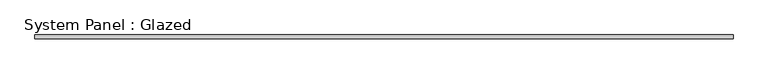
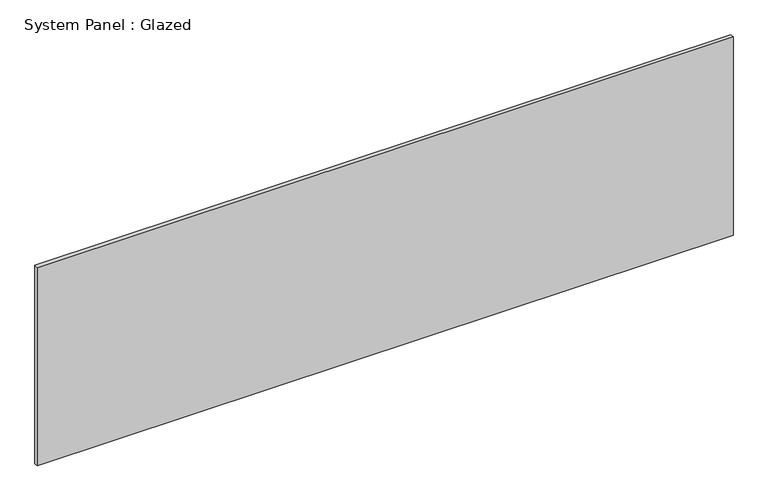
"""IFC4 building model written with IfcOpenShell, lengths in millimetres: plate geometry, System Panel : Glazed."""

from ifc_helpers import new_model, si_unit, origin, origin_with_axes, place, context, project, spatial, polyline, outline, extrude, source, transform, mapped, element, save


def system_panel_glazed_a32a2426(model_context):
    return source(origin(), model_context, "Body", "SweptSolid", [
        extrude(outline(polyline([(2425.7, 19.05), (-2425.7, 19.05), (-2425.7, 44.45), (2425.7, 44.45), (2425.7, 19.05)])), origin_with_axes(), (0.0, 0.0, 1.0), 1460.5),
    ])


if __name__ == "__main__":
    model = new_model("IFC4")
    model_context = context("Model", 3, world=origin())
    ifc_project = project(units=[si_unit("LENGTHUNIT", "METRE", prefix="MILLI")], contexts=[model_context])
    site = spatial("IfcSite", under=ifc_project)
    building = spatial("IfcBuilding", under=site)
    placement = place(None, origin())
    system_panel_glazed_shape = system_panel_glazed_a32a2426(model_context)
    element("IfcPlate", 1, ObjectType="System Panel : Glazed", at=placement, inside=building, context=model_context, shape_type="MappedRepresentation", body=[
        mapped(system_panel_glazed_shape, transform((0.0, 0.0, 0.0), x_axis=(1.0, 0.0, 0.0), y_axis=(0.0, 1.0, 0.0), z_axis=(0.0, 0.0, 1.0))),
    ])
    save(model, "model.ifc")

# Revit data of these elements
# Type "System Panel : Glazed"
#   Construction Type Id = "GSP4R"
#   Analytic Construction = "1/8 in Pilkington single glazing"
#   Visual Light Transmittance = 0.9
#   Solar Heat Gain Coefficient = 0.86
#   Heat Transfer Coefficient (U) = 1.18115 BTU/(h·ft²·°F)
# Element 1 (IfcPlate, "System Panel : Glazed")
#   Materials on its faces: "Glass"
# Materials
#   "Glass": class "Glass", colour RGB 0 128 192, transparency 0.75, Description = "Soda Lime Glass", Cost = 0
